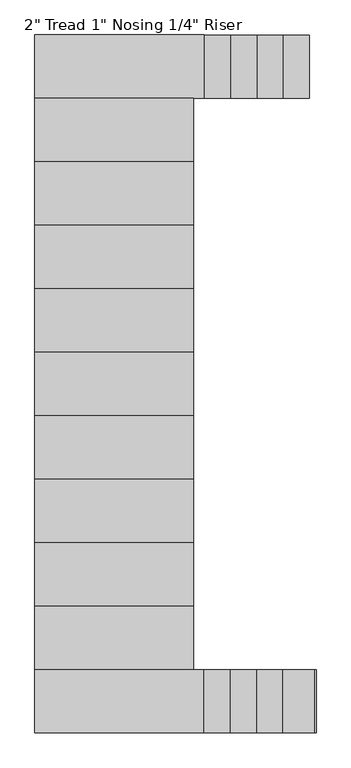
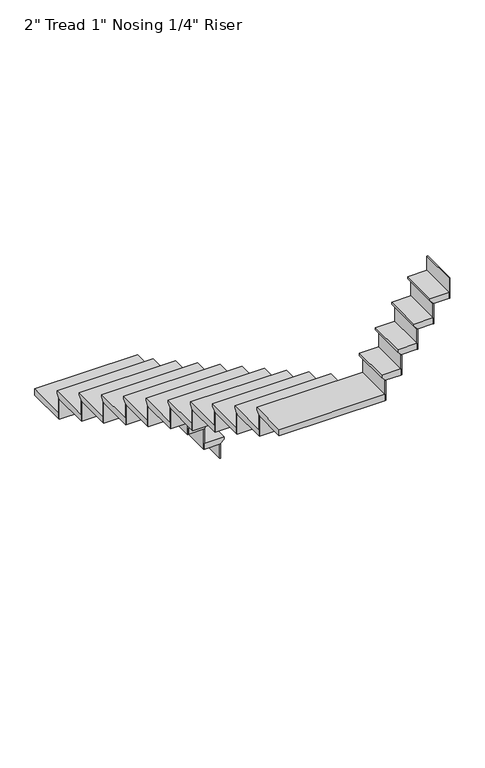
"""IFC4 building model written with IfcOpenShell, lengths in millimetres: stair flight geometry."""

from ifc_helpers import new_model, si_unit, origin, place, context, project, spatial, faceted_brep, source, transform, mapped, element, save


def stair_flight_0c8a4d61(model_context):
    return source(origin(), model_context, "Body", "Brep", [
        faceted_brep([(3073.4, 5613.4, 150.2833333), (3073.4, 5613.4, 169.3333333), (3073.4, 5308.6, 169.3333333), (3073.4, 5308.6, 150.2833333), (3048.0, 5613.4, 124.8833333), (3048.0, 5308.6, 124.8833333), (2921.0, 5613.4, 169.3333333), (2921.0, 5308.6, 169.3333333), (3048.0, 5308.6, 118.5333333), (2921.0, 5308.6, 118.5333333), (2921.0, 5613.4, 118.5333333), (3048.0, 5613.4, 118.5333333)], [[[0, 1, 2, 3]], [[4, 0, 3, 5]], [[2, 1, 6, 7]], [[8, 9, 10, 11]], [[2, 7, 9, 8, 5, 3]], [[8, 11, 4, 5]], [[6, 1, 0, 4, 11, 10]], [[7, 6, 10, 9]]]),
        faceted_brep([(3048.0, 5613.4, 118.5333333), (3048.0, 5613.4, 0.0), (3041.65, 5613.4, 0.0), (3041.65, 5613.4, 118.5333333), (3048.0, 5308.6, 118.5333333), (3041.65, 5308.6, 118.5333333), (3041.65, 5308.6, 0.0), (3048.0, 5308.6, 0.0)], [[[0, 1, 2, 3]], [[4, 5, 6, 7]], [[1, 0, 4, 7]], [[2, 1, 7, 6]], [[3, 2, 6, 5]], [[0, 3, 5, 4]]]),
        faceted_brep([(2921.0, 5613.4, 287.8666667), (2921.0, 5613.4, 118.5333333), (2914.65, 5613.4, 118.5333333), (2914.65, 5613.4, 287.8666667), (2921.0, 5308.6, 287.8666667), (2914.65, 5308.6, 287.8666667), (2914.65, 5308.6, 118.5333333), (2921.0, 5308.6, 118.5333333)], [[[0, 1, 2, 3]], [[4, 5, 6, 7]], [[1, 0, 4, 7]], [[2, 1, 7, 6]], [[3, 2, 6, 5]], [[0, 3, 5, 4]]]),
        faceted_brep([(2946.4, 5308.6, 338.6666667), (2946.4, 5613.4, 338.6666667), (2794.0, 5613.4, 338.6666667), (2794.0, 5308.6, 338.6666667), (2921.0, 5308.6, 287.8666667), (2794.0, 5308.6, 287.8666667), (2794.0, 5613.4, 287.8666667), (2921.0, 5613.4, 287.8666667), (2921.0, 5308.6, 294.2166667), (2946.4, 5308.6, 319.6166667), (2921.0, 5613.4, 294.2166667), (2946.4, 5613.4, 319.6166667)], [[[0, 1, 2, 3]], [[4, 5, 6, 7]], [[0, 3, 5, 4, 8, 9]], [[4, 7, 10, 8]], [[2, 1, 11, 10, 7, 6]], [[3, 2, 6, 5]], [[11, 1, 0, 9]], [[10, 11, 9, 8]]]),
        faceted_brep([(2794.0, 5613.4, 457.2), (2794.0, 5613.4, 287.8666667), (2787.65, 5613.4, 287.8666667), (2787.65, 5613.4, 457.2), (2794.0, 5308.6, 457.2), (2787.65, 5308.6, 457.2), (2787.65, 5308.6, 287.8666667), (2794.0, 5308.6, 287.8666667)], [[[0, 1, 2, 3]], [[4, 5, 6, 7]], [[1, 0, 4, 7]], [[2, 1, 7, 6]], [[3, 2, 6, 5]], [[0, 3, 5, 4]]]),
        faceted_brep([(2819.4, 5308.6, 508.0), (2819.4, 5613.4, 508.0), (2667.0, 5613.4, 508.0), (2667.0, 5308.6, 508.0), (2794.0, 5308.6, 457.2), (2667.0, 5308.6, 457.2), (2667.0, 5613.4, 457.2), (2794.0, 5613.4, 457.2), (2794.0, 5308.6, 463.55), (2819.4, 5308.6, 488.95), (2794.0, 5613.4, 463.55), (2819.4, 5613.4, 488.95)], [[[0, 1, 2, 3]], [[4, 5, 6, 7]], [[0, 3, 5, 4, 8, 9]], [[4, 7, 10, 8]], [[2, 1, 11, 10, 7, 6]], [[3, 2, 6, 5]], [[11, 1, 0, 9]], [[10, 11, 9, 8]]]),
        faceted_brep([(2667.0, 5613.4, 626.5333333), (2667.0, 5613.4, 457.2), (2660.65, 5613.4, 457.2), (2660.65, 5613.4, 626.5333333), (2667.0, 5308.6, 626.5333333), (2660.65, 5308.6, 626.5333333), (2660.65, 5308.6, 457.2), (2667.0, 5308.6, 457.2)], [[[0, 1, 2, 3]], [[4, 5, 6, 7]], [[1, 0, 4, 7]], [[2, 1, 7, 6]], [[3, 2, 6, 5]], [[0, 3, 5, 4]]]),
        faceted_brep([(2692.4, 5308.6, 677.3333333), (2692.4, 5613.4, 677.3333333), (2540.0, 5613.4, 677.3333333), (2540.0, 5308.6, 677.3333333), (2667.0, 5308.6, 626.5333333), (2540.0, 5308.6, 626.5333333), (2540.0, 5613.4, 626.5333333), (2667.0, 5613.4, 626.5333333), (2667.0, 5308.6, 632.8833333), (2692.4, 5308.6, 658.2833333), (2667.0, 5613.4, 632.8833333), (2692.4, 5613.4, 658.2833333)], [[[0, 1, 2, 3]], [[4, 5, 6, 7]], [[0, 3, 5, 4, 8, 9]], [[4, 7, 10, 8]], [[2, 1, 11, 10, 7, 6]], [[3, 2, 6, 5]], [[11, 1, 0, 9]], [[10, 11, 9, 8]]]),
        faceted_brep([(2540.0, 5613.4, 795.8666667), (2540.0, 5613.4, 626.5333333), (2533.65, 5613.4, 626.5333333), (2533.65, 5613.4, 795.8666667), (2540.0, 5308.6, 795.8666667), (2533.65, 5308.6, 795.8666667), (2533.65, 5308.6, 626.5333333), (2540.0, 5308.6, 626.5333333)], [[[0, 1, 2, 3]], [[4, 5, 6, 7]], [[1, 0, 4, 7]], [[2, 1, 7, 6]], [[3, 2, 6, 5]], [[0, 3, 5, 4]]]),
        faceted_brep([(2514.6, 5283.2, 846.6666667), (2514.6, 5308.6, 846.6666667), (2565.4, 5308.6, 846.6666667), (2565.4, 5613.4, 846.6666667), (1752.6, 5613.4, 846.6666667), (1752.6, 5283.2, 846.6666667), (2514.6, 5308.6, 795.8666667), (2514.6, 5283.2, 795.8666667), (1752.6, 5283.2, 795.8666667), (1752.6, 5613.4, 795.8666667), (2540.0, 5613.4, 795.8666667), (2540.0, 5308.6, 795.8666667), (2540.0, 5308.6, 802.2166667), (2565.4, 5308.6, 827.6166667), (2540.0, 5613.4, 802.2166667), (2565.4, 5613.4, 827.6166667)], [[[0, 1, 2, 3, 4, 5]], [[6, 7, 8, 9, 10, 11]], [[1, 0, 7, 6]], [[2, 1, 6, 11, 12, 13]], [[11, 10, 14, 12]], [[4, 3, 15, 14, 10, 9]], [[5, 4, 9, 8]], [[0, 5, 8, 7]], [[15, 3, 2, 13]], [[14, 15, 13, 12]]]),
        faceted_brep([(1752.6, 5283.2, 965.2), (1752.6, 5283.2, 795.8666667), (1752.6, 5276.85, 795.8666667), (1752.6, 5276.85, 965.2), (2514.6, 5283.2, 965.2), (2514.6, 5276.85, 965.2), (2514.6, 5276.85, 795.8666667), (2514.6, 5283.2, 795.8666667)], [[[0, 1, 2, 3]], [[4, 5, 6, 7]], [[1, 0, 4, 7]], [[2, 1, 7, 6]], [[3, 2, 6, 5]], [[0, 3, 5, 4]]]),
        faceted_brep([(2514.6, 5308.6, 1016.0), (1752.6, 5308.6, 1016.0), (1752.6, 4978.4, 1016.0), (2514.6, 4978.4, 1016.0), (2514.6, 5283.2, 965.2), (2514.6, 4978.4, 965.2), (1752.6, 4978.4, 965.2), (1752.6, 5283.2, 965.2), (2514.6, 5283.2, 971.55), (2514.6, 5308.6, 996.95), (1752.6, 5283.2, 971.55), (1752.6, 5308.6, 996.95)], [[[0, 1, 2, 3]], [[4, 5, 6, 7]], [[0, 3, 5, 4, 8, 9]], [[4, 7, 10, 8]], [[2, 1, 11, 10, 7, 6]], [[3, 2, 6, 5]], [[11, 1, 0, 9]], [[10, 11, 9, 8]]]),
        faceted_brep([(1752.6, 4978.4, 1134.5333333), (1752.6, 4978.4, 965.2), (1752.6, 4972.05, 965.2), (1752.6, 4972.05, 1134.5333333), (2514.6, 4978.4, 1134.5333333), (2514.6, 4972.05, 1134.5333333), (2514.6, 4972.05, 965.2), (2514.6, 4978.4, 965.2)], [[[0, 1, 2, 3]], [[4, 5, 6, 7]], [[1, 0, 4, 7]], [[2, 1, 7, 6]], [[3, 2, 6, 5]], [[0, 3, 5, 4]]]),
        faceted_brep([(2514.6, 5003.8, 1185.3333333), (1752.6, 5003.8, 1185.3333333), (1752.6, 4673.6, 1185.3333333), (2514.6, 4673.6, 1185.3333333), (2514.6, 4978.4, 1134.5333333), (2514.6, 4673.6, 1134.5333333), (1752.6, 4673.6, 1134.5333333), (1752.6, 4978.4, 1134.5333333), (2514.6, 4978.4, 1140.8833333), (2514.6, 5003.8, 1166.2833333), (1752.6, 4978.4, 1140.8833333), (1752.6, 5003.8, 1166.2833333)], [[[0, 1, 2, 3]], [[4, 5, 6, 7]], [[0, 3, 5, 4, 8, 9]], [[4, 7, 10, 8]], [[2, 1, 11, 10, 7, 6]], [[3, 2, 6, 5]], [[11, 1, 0, 9]], [[10, 11, 9, 8]]]),
        faceted_brep([(1752.6, 4673.6, 1303.8666667), (1752.6, 4673.6, 1134.5333333), (1752.6, 4667.25, 1134.5333333), (1752.6, 4667.25, 1303.8666667), (2514.6, 4673.6, 1303.8666667), (2514.6, 4667.25, 1303.8666667), (2514.6, 4667.25, 1134.5333333), (2514.6, 4673.6, 1134.5333333)], [[[0, 1, 2, 3]], [[4, 5, 6, 7]], [[1, 0, 4, 7]], [[2, 1, 7, 6]], [[3, 2, 6, 5]], [[0, 3, 5, 4]]]),
        faceted_brep([(2514.6, 4699.0, 1354.6666667), (1752.6, 4699.0, 1354.6666667), (1752.6, 4368.8, 1354.6666667), (2514.6, 4368.8, 1354.6666667), (2514.6, 4673.6, 1303.8666667), (2514.6, 4368.8, 1303.8666667), (1752.6, 4368.8, 1303.8666667), (1752.6, 4673.6, 1303.8666667), (2514.6, 4673.6, 1310.2166667), (2514.6, 4699.0, 1335.6166667), (1752.6, 4673.6, 1310.2166667), (1752.6, 4699.0, 1335.6166667)], [[[0, 1, 2, 3]], [[4, 5, 6, 7]], [[0, 3, 5, 4, 8, 9]], [[4, 7, 10, 8]], [[2, 1, 11, 10, 7, 6]], [[3, 2, 6, 5]], [[11, 1, 0, 9]], [[10, 11, 9, 8]]]),
        faceted_brep([(1752.6, 4368.8, 1473.2), (1752.6, 4368.8, 1303.8666667), (1752.6, 4362.45, 1303.8666667), (1752.6, 4362.45, 1473.2), (2514.6, 4368.8, 1473.2), (2514.6, 4362.45, 1473.2), (2514.6, 4362.45, 1303.8666667), (2514.6, 4368.8, 1303.8666667)], [[[0, 1, 2, 3]], [[4, 5, 6, 7]], [[1, 0, 4, 7]], [[2, 1, 7, 6]], [[3, 2, 6, 5]], [[0, 3, 5, 4]]]),
        faceted_brep([(2514.6, 4394.2, 1524.0), (1752.6, 4394.2, 1524.0), (1752.6, 4064.0, 1524.0), (2514.6, 4064.0, 1524.0), (2514.6, 4368.8, 1473.2), (2514.6, 4064.0, 1473.2), (1752.6, 4064.0, 1473.2), (1752.6, 4368.8, 1473.2), (2514.6, 4368.8, 1479.55), (2514.6, 4394.2, 1504.95), (1752.6, 4368.8, 1479.55), (1752.6, 4394.2, 1504.95)], [[[0, 1, 2, 3]], [[4, 5, 6, 7]], [[0, 3, 5, 4, 8, 9]], [[4, 7, 10, 8]], [[2, 1, 11, 10, 7, 6]], [[3, 2, 6, 5]], [[11, 1, 0, 9]], [[10, 11, 9, 8]]]),
        faceted_brep([(1752.6, 4064.0, 1642.5333333), (1752.6, 4064.0, 1473.2), (1752.6, 4057.65, 1473.2), (1752.6, 4057.65, 1642.5333333), (2514.6, 4064.0, 1642.5333333), (2514.6, 4057.65, 1642.5333333), (2514.6, 4057.65, 1473.2), (2514.6, 4064.0, 1473.2)], [[[0, 1, 2, 3]], [[4, 5, 6, 7]], [[1, 0, 4, 7]], [[2, 1, 7, 6]], [[3, 2, 6, 5]], [[0, 3, 5, 4]]]),
        faceted_brep([(2514.6, 4089.4, 1693.3333333), (1752.6, 4089.4, 1693.3333333), (1752.6, 3759.2, 1693.3333333), (2514.6, 3759.2, 1693.3333333), (2514.6, 4064.0, 1642.5333333), (2514.6, 3759.2, 1642.5333333), (1752.6, 3759.2, 1642.5333333), (1752.6, 4064.0, 1642.5333333), (2514.6, 4064.0, 1648.8833333), (2514.6, 4089.4, 1674.2833333), (1752.6, 4064.0, 1648.8833333), (1752.6, 4089.4, 1674.2833333)], [[[0, 1, 2, 3]], [[4, 5, 6, 7]], [[0, 3, 5, 4, 8, 9]], [[4, 7, 10, 8]], [[2, 1, 11, 10, 7, 6]], [[3, 2, 6, 5]], [[11, 1, 0, 9]], [[10, 11, 9, 8]]]),
        faceted_brep([(1752.6, 3759.2, 1811.8666667), (1752.6, 3759.2, 1642.5333333), (1752.6, 3752.85, 1642.5333333), (1752.6, 3752.85, 1811.8666667), (2514.6, 3759.2, 1811.8666667), (2514.6, 3752.85, 1811.8666667), (2514.6, 3752.85, 1642.5333333), (2514.6, 3759.2, 1642.5333333)], [[[0, 1, 2, 3]], [[4, 5, 6, 7]], [[1, 0, 4, 7]], [[2, 1, 7, 6]], [[3, 2, 6, 5]], [[0, 3, 5, 4]]]),
        faceted_brep([(2514.6, 3784.6, 1862.6666667), (1752.6, 3784.6, 1862.6666667), (1752.6, 3454.4, 1862.6666667), (2514.6, 3454.4, 1862.6666667), (2514.6, 3759.2, 1811.8666667), (2514.6, 3454.4, 1811.8666667), (1752.6, 3454.4, 1811.8666667), (1752.6, 3759.2, 1811.8666667), (2514.6, 3759.2, 1818.2166667), (2514.6, 3784.6, 1843.6166667), (1752.6, 3759.2, 1818.2166667), (1752.6, 3784.6, 1843.6166667)], [[[0, 1, 2, 3]], [[4, 5, 6, 7]], [[0, 3, 5, 4, 8, 9]], [[4, 7, 10, 8]], [[2, 1, 11, 10, 7, 6]], [[3, 2, 6, 5]], [[11, 1, 0, 9]], [[10, 11, 9, 8]]]),
        faceted_brep([(1752.6, 3454.4, 1981.2), (1752.6, 3454.4, 1811.8666667), (1752.6, 3448.05, 1811.8666667), (1752.6, 3448.05, 1981.2), (2514.6, 3454.4, 1981.2), (2514.6, 3448.05, 1981.2), (2514.6, 3448.05, 1811.8666667), (2514.6, 3454.4, 1811.8666667)], [[[0, 1, 2, 3]], [[4, 5, 6, 7]], [[1, 0, 4, 7]], [[2, 1, 7, 6]], [[3, 2, 6, 5]], [[0, 3, 5, 4]]]),
        faceted_brep([(2514.6, 3479.8, 2032.0), (1752.6, 3479.8, 2032.0), (1752.6, 3149.6, 2032.0), (2514.6, 3149.6, 2032.0), (2514.6, 3454.4, 1981.2), (2514.6, 3149.6, 1981.2), (1752.6, 3149.6, 1981.2), (1752.6, 3454.4, 1981.2), (2514.6, 3454.4, 1987.55), (2514.6, 3479.8, 2012.95), (1752.6, 3454.4, 1987.55), (1752.6, 3479.8, 2012.95)], [[[0, 1, 2, 3]], [[4, 5, 6, 7]], [[0, 3, 5, 4, 8, 9]], [[4, 7, 10, 8]], [[2, 1, 11, 10, 7, 6]], [[3, 2, 6, 5]], [[11, 1, 0, 9]], [[10, 11, 9, 8]]]),
        faceted_brep([(1752.6, 3149.6, 2150.5333333), (1752.6, 3149.6, 1981.2), (1752.6, 3143.25, 1981.2), (1752.6, 3143.25, 2150.5333333), (2514.6, 3149.6, 2150.5333333), (2514.6, 3143.25, 2150.5333333), (2514.6, 3143.25, 1981.2), (2514.6, 3149.6, 1981.2)], [[[0, 1, 2, 3]], [[4, 5, 6, 7]], [[1, 0, 4, 7]], [[2, 1, 7, 6]], [[3, 2, 6, 5]], [[0, 3, 5, 4]]]),
        faceted_brep([(2514.6, 3175.0, 2201.3333333), (1752.6, 3175.0, 2201.3333333), (1752.6, 2844.8, 2201.3333333), (2514.6, 2844.8, 2201.3333333), (2514.6, 3149.6, 2150.5333333), (2514.6, 2844.8, 2150.5333333), (1752.6, 2844.8, 2150.5333333), (1752.6, 3149.6, 2150.5333333), (2514.6, 3149.6, 2156.8833333), (2514.6, 3175.0, 2182.2833333), (1752.6, 3149.6, 2156.8833333), (1752.6, 3175.0, 2182.2833333)], [[[0, 1, 2, 3]], [[4, 5, 6, 7]], [[0, 3, 5, 4, 8, 9]], [[4, 7, 10, 8]], [[2, 1, 11, 10, 7, 6]], [[3, 2, 6, 5]], [[11, 1, 0, 9]], [[10, 11, 9, 8]]]),
        faceted_brep([(1752.6, 2844.8, 2319.8666667), (1752.6, 2844.8, 2150.5333333), (1752.6, 2838.45, 2150.5333333), (1752.6, 2838.45, 2319.8666667), (2514.6, 2844.8, 2319.8666667), (2514.6, 2838.45, 2319.8666667), (2514.6, 2838.45, 2150.5333333), (2514.6, 2844.8, 2150.5333333)], [[[0, 1, 2, 3]], [[4, 5, 6, 7]], [[1, 0, 4, 7]], [[2, 1, 7, 6]], [[3, 2, 6, 5]], [[0, 3, 5, 4]]]),
        faceted_brep([(2514.6, 2870.2, 2370.6666667), (1752.6, 2870.2, 2370.6666667), (1752.6, 2540.0, 2370.6666667), (2514.6, 2540.0, 2370.6666667), (2514.6, 2844.8, 2319.8666667), (2514.6, 2540.0, 2319.8666667), (1752.6, 2540.0, 2319.8666667), (1752.6, 2844.8, 2319.8666667), (2514.6, 2844.8, 2326.2166667), (2514.6, 2870.2, 2351.6166667), (1752.6, 2844.8, 2326.2166667), (1752.6, 2870.2, 2351.6166667)], [[[0, 1, 2, 3]], [[4, 5, 6, 7]], [[0, 3, 5, 4, 8, 9]], [[4, 7, 10, 8]], [[2, 1, 11, 10, 7, 6]], [[3, 2, 6, 5]], [[11, 1, 0, 9]], [[10, 11, 9, 8]]]),
        faceted_brep([(1752.6, 2540.0, 2489.2), (1752.6, 2540.0, 2319.8666667), (1752.6, 2533.65, 2319.8666667), (1752.6, 2533.65, 2489.2), (2514.6, 2540.0, 2489.2), (2514.6, 2533.65, 2489.2), (2514.6, 2533.65, 2319.8666667), (2514.6, 2540.0, 2319.8666667)], [[[0, 1, 2, 3]], [[4, 5, 6, 7]], [[1, 0, 4, 7]], [[2, 1, 7, 6]], [[3, 2, 6, 5]], [[0, 3, 5, 4]]]),
        faceted_brep([(1752.6, 2260.6, 2540.0), (2590.8, 2260.6, 2540.0), (2590.8, 2565.4, 2540.0), (1752.6, 2565.4, 2540.0), (2514.6, 2565.4, 2489.2), (2590.8, 2565.4, 2489.2), (2590.8, 2260.6, 2489.2), (1752.6, 2260.6, 2489.2), (1752.6, 2540.0, 2489.2), (2514.6, 2540.0, 2489.2), (2514.6, 2565.4, 2520.95), (1752.6, 2565.4, 2520.95), (2514.6, 2540.0, 2495.55), (1752.6, 2540.0, 2495.55)], [[[0, 1, 2, 3]], [[4, 5, 6, 7, 8, 9]], [[3, 2, 5, 4, 10, 11]], [[4, 9, 12, 10]], [[9, 8, 13, 12]], [[0, 3, 11, 13, 8, 7]], [[1, 0, 7, 6]], [[2, 1, 6, 5]], [[13, 11, 10, 12]]]),
        faceted_brep([(2590.8, 2260.6, 2658.5333333), (2590.8, 2260.6, 2489.2), (2597.15, 2260.6, 2489.2), (2597.15, 2260.6, 2658.5333333), (2590.8, 2565.4, 2658.5333333), (2597.15, 2565.4, 2658.5333333), (2597.15, 2565.4, 2489.2), (2590.8, 2565.4, 2489.2)], [[[0, 1, 2, 3]], [[4, 5, 6, 7]], [[1, 0, 4, 7]], [[2, 1, 7, 6]], [[3, 2, 6, 5]], [[0, 3, 5, 4]]]),
        faceted_brep([(2565.4, 2565.4, 2709.3333333), (2565.4, 2260.6, 2709.3333333), (2717.8, 2260.6, 2709.3333333), (2717.8, 2565.4, 2709.3333333), (2590.8, 2565.4, 2658.5333333), (2717.8, 2565.4, 2658.5333333), (2717.8, 2260.6, 2658.5333333), (2590.8, 2260.6, 2658.5333333), (2590.8, 2565.4, 2664.8833333), (2565.4, 2565.4, 2690.2833333), (2590.8, 2260.6, 2664.8833333), (2565.4, 2260.6, 2690.2833333)], [[[0, 1, 2, 3]], [[4, 5, 6, 7]], [[0, 3, 5, 4, 8, 9]], [[4, 7, 10, 8]], [[2, 1, 11, 10, 7, 6]], [[3, 2, 6, 5]], [[11, 1, 0, 9]], [[10, 11, 9, 8]]]),
        faceted_brep([(2717.8, 2260.6, 2827.8666667), (2717.8, 2260.6, 2658.5333333), (2724.15, 2260.6, 2658.5333333), (2724.15, 2260.6, 2827.8666667), (2717.8, 2565.4, 2827.8666667), (2724.15, 2565.4, 2827.8666667), (2724.15, 2565.4, 2658.5333333), (2717.8, 2565.4, 2658.5333333)], [[[0, 1, 2, 3]], [[4, 5, 6, 7]], [[1, 0, 4, 7]], [[2, 1, 7, 6]], [[3, 2, 6, 5]], [[0, 3, 5, 4]]]),
        faceted_brep([(2692.4, 2565.4, 2878.6666667), (2692.4, 2260.6, 2878.6666667), (2844.8, 2260.6, 2878.6666667), (2844.8, 2565.4, 2878.6666667), (2717.8, 2565.4, 2827.8666667), (2844.8, 2565.4, 2827.8666667), (2844.8, 2260.6, 2827.8666667), (2717.8, 2260.6, 2827.8666667), (2717.8, 2565.4, 2834.2166667), (2692.4, 2565.4, 2859.6166667), (2717.8, 2260.6, 2834.2166667), (2692.4, 2260.6, 2859.6166667)], [[[0, 1, 2, 3]], [[4, 5, 6, 7]], [[0, 3, 5, 4, 8, 9]], [[4, 7, 10, 8]], [[2, 1, 11, 10, 7, 6]], [[3, 2, 6, 5]], [[11, 1, 0, 9]], [[10, 11, 9, 8]]]),
        faceted_brep([(2844.8, 2260.6, 2997.2), (2844.8, 2260.6, 2827.8666667), (2851.15, 2260.6, 2827.8666667), (2851.15, 2260.6, 2997.2), (2844.8, 2565.4, 2997.2), (2851.15, 2565.4, 2997.2), (2851.15, 2565.4, 2827.8666667), (2844.8, 2565.4, 2827.8666667)], [[[0, 1, 2, 3]], [[4, 5, 6, 7]], [[1, 0, 4, 7]], [[2, 1, 7, 6]], [[3, 2, 6, 5]], [[0, 3, 5, 4]]]),
        faceted_brep([(2819.4, 2565.4, 3048.0), (2819.4, 2260.6, 3048.0), (2971.8, 2260.6, 3048.0), (2971.8, 2565.4, 3048.0), (2844.8, 2565.4, 2997.2), (2971.8, 2565.4, 2997.2), (2971.8, 2260.6, 2997.2), (2844.8, 2260.6, 2997.2), (2844.8, 2565.4, 3003.55), (2819.4, 2565.4, 3028.95), (2844.8, 2260.6, 3003.55), (2819.4, 2260.6, 3028.95)], [[[0, 1, 2, 3]], [[4, 5, 6, 7]], [[0, 3, 5, 4, 8, 9]], [[4, 7, 10, 8]], [[2, 1, 11, 10, 7, 6]], [[3, 2, 6, 5]], [[11, 1, 0, 9]], [[10, 11, 9, 8]]]),
        faceted_brep([(2971.8, 2260.6, 3166.5333333), (2971.8, 2260.6, 2997.2), (2978.15, 2260.6, 2997.2), (2978.15, 2260.6, 3166.5333333), (2971.8, 2565.4, 3166.5333333), (2978.15, 2565.4, 3166.5333333), (2978.15, 2565.4, 2997.2), (2971.8, 2565.4, 2997.2)], [[[0, 1, 2, 3]], [[4, 5, 6, 7]], [[1, 0, 4, 7]], [[2, 1, 7, 6]], [[3, 2, 6, 5]], [[0, 3, 5, 4]]]),
        faceted_brep([(3098.8, 2260.6, 3335.8666667), (3098.8, 2260.6, 3166.5333333), (3105.15, 2260.6, 3166.5333333), (3105.15, 2260.6, 3335.8666667), (3098.8, 2565.4, 3335.8666667), (3105.15, 2565.4, 3335.8666667), (3105.15, 2565.4, 3166.5333333), (3098.8, 2565.4, 3166.5333333)], [[[0, 1, 2, 3]], [[4, 5, 6, 7]], [[1, 0, 4, 7]], [[2, 1, 7, 6]], [[3, 2, 6, 5]], [[0, 3, 5, 4]]]),
        faceted_brep([(2946.4, 2565.4, 3217.3333333), (2946.4, 2260.6, 3217.3333333), (3098.8, 2260.6, 3217.3333333), (3098.8, 2565.4, 3217.3333333), (2971.8, 2565.4, 3166.5333333), (3098.8, 2565.4, 3166.5333333), (3098.8, 2260.6, 3166.5333333), (2971.8, 2260.6, 3166.5333333), (2971.8, 2565.4, 3172.8833333), (2946.4, 2565.4, 3198.2833333), (2971.8, 2260.6, 3172.8833333), (2946.4, 2260.6, 3198.2833333)], [[[0, 1, 2, 3]], [[4, 5, 6, 7]], [[0, 3, 5, 4, 8, 9]], [[4, 7, 10, 8]], [[2, 1, 11, 10, 7, 6]], [[3, 2, 6, 5]], [[11, 1, 0, 9]], [[10, 11, 9, 8]]]),
    ])


if __name__ == "__main__":
    model = new_model("IFC4")
    model_context = context("Model", 3, world=origin())
    ifc_project = project(units=[si_unit("LENGTHUNIT", "METRE", prefix="MILLI")], contexts=[model_context])
    site = spatial("IfcSite", under=ifc_project)
    building = spatial("IfcBuilding", under=site)
    placement = place(None, origin())
    stair_flight_shape = stair_flight_0c8a4d61(model_context)
    element("IfcStairFlight", 1, ObjectType="2\" Tread 1\" Nosing 1/4\" Riser", at=placement, inside=building, context=model_context, shape_type="MappedRepresentation", body=[
        mapped(stair_flight_shape, transform((0.0, 0.0, 0.0), x_axis=(1.0, 0.0, 0.0), y_axis=(0.0, 1.0, 0.0), z_axis=(0.0, 0.0, 1.0))),
    ])
    save(model, "model.ifc")
